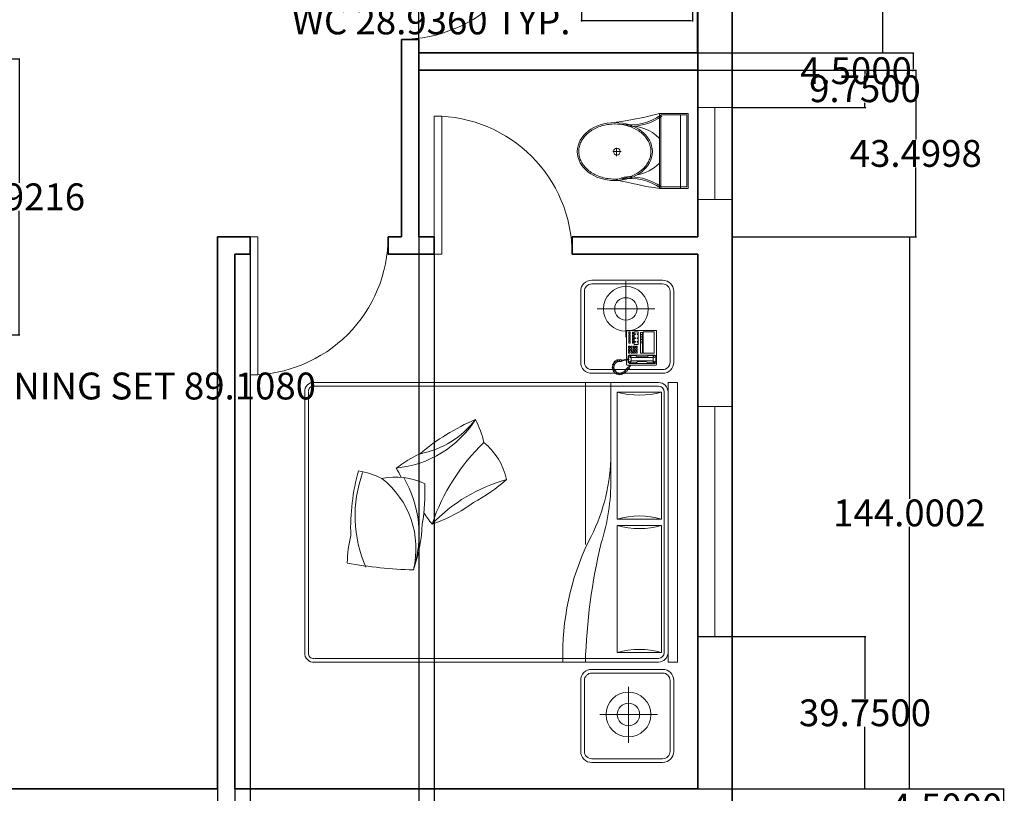
# Model space of a CAD drawing. Units: inches. Extents: x 774 to 2194, y 522 to 1247.
# Tile 3 of 7: x 1035 to 1292, y 668 to 870. Entities that reach past the tile are written whole.
import ezdxf

# ---------------------------------------------------------------- set-up
doc = ezdxf.new("R2010")
doc.units = ezdxf.units.IN
for name, color, linetype, lineweight in [('A-ANNO-DIMS', 2, 'Continuous', 13), ('A-DOOR', 3, 'Continuous', 18), ('A-FLOR-FIXT', 7, 'Continuous', 18), ('A-FURN', 8, 'Continuous', 18), ('A-GLAZ', 4, 'Continuous', 18), ('A-WALL', 7, 'Continuous', 35)]:
    doc.layers.add(name, color=color, linetype=linetype, lineweight=lineweight)
doc.styles.get("Standard").update_dxf_attribs({"font": 'arial.ttf'})
doc.dimstyles.get("Standard").update_dxf_attribs({"dimtxt": 7, "dimasz": 0.18, "dimexe": 0.18, "dimexo": 0.0625, "dimgap": 0.09, "dimtad": 0, "dimtih": 1, "dimtoh": 1, "dimdec": 4, "dimzin": 0, "dimdsep": 46, "dimtxsty": 'Standard', "dimcen": 0.09, "dimadec": 0, "dimazin": 0, "dimtfac": 1, "dimtdec": 4, "dimtofl": 0, "dimtmove": 0, "dimatfit": 3, "dimfxl": 1, "dimtolj": 1, "dimtzin": 0, "dimarcsym": 0})

# ---------------------------------------------------------------- blocks, each defined once
blk = doc.blocks.new('A$C356F0359')
for p, q in [((0.4398, 1.9801), (0.0598, 1.9801)), ((0.4398, 1.9601), (0.0598, 1.9601)), ((0.5489, 2), (2.0492, 2)), ((0.5489, 1.9489), (0.5489, 2)), ((2.0492, 1.9489), (2.0492, 2)), ((2.5283, 1.9801), (2.1483, 1.9801)), ((2.5283, 1.9601), (2.1483, 1.9601)), ((-0.0002, 1.9201), (-0.0002, 1.5401)), ((0.0198, 1.9201), (0.0198, 1.5401)), ((0.4798, 1.5401), (0.4798, 1.9201)), ((0.4998, 1.5401), (0.4998, 1.9201)), ((2.0492, 1.9489), (0.5489, 1.9489)), ((1.998, 1.9289), (0.6001, 1.9289)), ((2.0883, 1.9201), (2.0883, 1.5401)), ((2.1083, 1.9201), (2.1083, 1.5401)), ((2.5683, 1.5401), (2.5683, 1.9201)), ((2.5883, 1.5401), (2.5883, 1.9201)), ((0.1539, 1.5681), (0.1539, 1.8777)), ((0.2725, 1.8879), (0.2702, 1.8856)), ((0.2702, 1.8856), (0.2702, 1.7279)), ((0.2725, 1.8879), (0.4531, 1.8879)), ((0.3913, 1.8753), (0.277, 1.8753)), ((0.277, 1.8753), (0.277, 1.8147)), ((0.3913, 1.8147), (0.3913, 1.8753)), ((0.4016, 1.8787), (0.4062, 1.8845)), ((0.4016, 1.7404), (0.4016, 1.8787)), ((0.4062, 1.881), (0.405, 1.8765)), ((0.405, 1.8765), (0.4153, 1.8662)), ((0.405, 1.8765), (0.405, 1.8456)), ((0.4062, 1.8845), (0.4405, 1.8845)), ((0.4108, 1.8833), (0.4062, 1.881)), ((0.4108, 1.8833), (0.4382, 1.8833)), ((0.4165, 1.8685), (0.4108, 1.8833)), ((0.4153, 1.8662), (0.4165, 1.8685)), ((0.4153, 1.8147), (0.4153, 1.8662)), ((0.4325, 1.8685), (0.4165, 1.8685)), ((0.4325, 1.8685), (0.4382, 1.8833)), ((0.4336, 1.8662), (0.4325, 1.8685)), ((0.4439, 1.8765), (0.4336, 1.8662)), ((0.4336, 1.8147), (0.4336, 1.8662)), ((0.4382, 1.8833), (0.4428, 1.881)), ((0.4405, 1.8845), (0.4462, 1.8787)), ((0.4428, 1.881), (0.4439, 1.8765)), ((0.4439, 1.8765), (0.4439, 1.8456)), ((0.4462, 1.8787), (0.4462, 1.7416)), ((0.4531, 1.8879), (0.4553, 1.8856)), ((0.4553, 1.8856), (0.4553, 1.7279)), ((0.5489, 1.8977), (0.5489, 0.0512)), ((0.5689, 1.8977), (0.5689, 0.0512)), ((2.0292, 0.0512), (2.0292, 1.8977)), ((2.0492, 0.0512), (2.0492, 1.8977)), ((2.3306, 1.5822), (2.3306, 1.8917)), ((0.277, 1.8147), (0.3913, 1.8147)), ((0.3913, 1.8125), (0.2816, 1.8125)), ((0.2816, 1.8125), (0.2816, 1.801)), ((0.2816, 1.801), (0.3913, 1.801)), ((0.2907, 1.8125), (0.2907, 1.801)), ((0.2999, 1.8125), (0.2999, 1.801)), ((0.309, 1.8125), (0.309, 1.801)), ((0.3182, 1.8125), (0.3182, 1.801)), ((0.3273, 1.8125), (0.3273, 1.801)), ((0.3365, 1.8125), (0.3365, 1.801)), ((0.3913, 1.801), (0.3913, 1.8125)), ((0.405, 1.8456), (0.4073, 1.8399)), ((0.4073, 1.8399), (0.4108, 1.8342)), ((0.4108, 1.8342), (0.4119, 1.8262)), ((0.4119, 1.8262), (0.4119, 1.8147)), ((0.4119, 1.793), (0.4119, 1.8147)), ((0.4153, 1.8147), (0.4153, 1.753)), ((0.4336, 1.8147), (0.4336, 1.753)), ((0.4382, 1.8342), (0.4371, 1.8262)), ((0.4371, 1.8262), (0.4371, 1.8147)), ((0.4371, 1.793), (0.4371, 1.8147)), ((0.4416, 1.8399), (0.4382, 1.8342)), ((0.4439, 1.8456), (0.4416, 1.8399)), ((0.277, 1.7885), (0.277, 1.7679)), ((0.3445, 1.7885), (0.277, 1.7885)), ((0.277, 1.7679), (0.3445, 1.7679)), ((0.2782, 1.7622), (0.2782, 1.7576)), ((0.2896, 1.7622), (0.2782, 1.7622)), ((0.2782, 1.7576), (0.2896, 1.7576)), ((0.2782, 1.745), (0.2896, 1.745)), ((0.2782, 1.7382), (0.2782, 1.745)), ((0.2885, 1.7862), (0.2885, 1.7827)), ((0.2919, 1.7862), (0.2885, 1.7862)), ((0.2885, 1.7827), (0.2919, 1.7827)), ((0.2919, 1.7736), (0.2885, 1.7736)), ((0.2885, 1.7736), (0.2885, 1.7702)), ((0.2885, 1.7702), (0.2919, 1.7702)), ((0.2896, 1.7576), (0.2896, 1.7622)), ((0.2896, 1.745), (0.2896, 1.7382)), ((0.2919, 1.7827), (0.2919, 1.7862)), ((0.2919, 1.7702), (0.2919, 1.7736)), ((0.2942, 1.7622), (0.2942, 1.7576)), ((0.3056, 1.7622), (0.2942, 1.7622)), ((0.2942, 1.7576), (0.3056, 1.7576)), ((0.2942, 1.745), (0.3056, 1.745)), ((0.2942, 1.7382), (0.2942, 1.745)), ((0.3056, 1.7576), (0.3056, 1.7622)), ((0.3056, 1.745), (0.3056, 1.7382)), ((0.3125, 1.7862), (0.309, 1.7862)), ((0.309, 1.7862), (0.309, 1.7827)), ((0.309, 1.7827), (0.3125, 1.7827)), ((0.3125, 1.7736), (0.309, 1.7736)), ((0.309, 1.7736), (0.309, 1.7702)), ((0.309, 1.7702), (0.3125, 1.7702)), ((0.3102, 1.7622), (0.3102, 1.7576)), ((0.3216, 1.7622), (0.3102, 1.7622)), ((0.3102, 1.7576), (0.3216, 1.7576)), ((0.3102, 1.745), (0.3216, 1.745)), ((0.3102, 1.7382), (0.3102, 1.745)), ((0.3125, 1.7827), (0.3125, 1.7862)), ((0.3125, 1.7702), (0.3125, 1.7736)), ((0.3216, 1.7576), (0.3216, 1.7622)), ((0.3216, 1.745), (0.3216, 1.7382)), ((0.3376, 1.7622), (0.3262, 1.7622)), ((0.3262, 1.7622), (0.3262, 1.7576)), ((0.3262, 1.7576), (0.3376, 1.7576)), ((0.3262, 1.7382), (0.3262, 1.745)), ((0.3262, 1.745), (0.3376, 1.745)), ((0.333, 1.7862), (0.3296, 1.7862)), ((0.3296, 1.7862), (0.3296, 1.7827)), ((0.3296, 1.7827), (0.333, 1.7827)), ((0.333, 1.7736), (0.3296, 1.7736)), ((0.3296, 1.7736), (0.3296, 1.7702)), ((0.3296, 1.7702), (0.333, 1.7702)), ((0.333, 1.7827), (0.333, 1.7862)), ((0.333, 1.7702), (0.333, 1.7736)), ((0.3376, 1.7576), (0.3376, 1.7622)), ((0.3376, 1.745), (0.3376, 1.7382)), ((0.3445, 1.7679), (0.3445, 1.7885)), ((0.3548, 1.7759), (0.3548, 1.7827)), ((0.3548, 1.7827), (0.3639, 1.7827)), ((0.3639, 1.7759), (0.3548, 1.7759)), ((0.3548, 1.7633), (0.3548, 1.7702)), ((0.3548, 1.7702), (0.3639, 1.7702)), ((0.3639, 1.7633), (0.3548, 1.7633)), ((0.3548, 1.7564), (0.3639, 1.7564)), ((0.3548, 1.7496), (0.3548, 1.7564)), ((0.3639, 1.7496), (0.3548, 1.7496)), ((0.3639, 1.7827), (0.3639, 1.7759)), ((0.3639, 1.7702), (0.3639, 1.7633)), ((0.3639, 1.7564), (0.3639, 1.7496)), ((0.3685, 1.7827), (0.3776, 1.7827)), ((0.3685, 1.7759), (0.3685, 1.7827)), ((0.3776, 1.7759), (0.3685, 1.7759)), ((0.3685, 1.7633), (0.3685, 1.7702)), ((0.3685, 1.7702), (0.3776, 1.7702)), ((0.3776, 1.7633), (0.3685, 1.7633)), ((0.3685, 1.7564), (0.3776, 1.7564)), ((0.3685, 1.7496), (0.3685, 1.7564)), ((0.3776, 1.7496), (0.3685, 1.7496)), ((0.3776, 1.7827), (0.3776, 1.7759)), ((0.3776, 1.7702), (0.3776, 1.7633)), ((0.3776, 1.7564), (0.3776, 1.7496)), ((0.3822, 1.7759), (0.3822, 1.7827)), ((0.3822, 1.7827), (0.3913, 1.7827)), ((0.3913, 1.7759), (0.3822, 1.7759)), ((0.3822, 1.7633), (0.3822, 1.7702)), ((0.3822, 1.7702), (0.3913, 1.7702)), ((0.3913, 1.7633), (0.3822, 1.7633)), ((0.3822, 1.7576), (0.3913, 1.7576)), ((0.3822, 1.7507), (0.3822, 1.7576)), ((0.3913, 1.7507), (0.3822, 1.7507)), ((0.3913, 1.7827), (0.3913, 1.7759)), ((0.3913, 1.7702), (0.3913, 1.7633)), ((0.3913, 1.7576), (0.3913, 1.7507)), ((0.405, 1.7736), (0.4073, 1.7793)), ((0.405, 1.7427), (0.405, 1.7736)), ((0.405, 1.7427), (0.4153, 1.753)), ((0.4073, 1.7793), (0.4108, 1.785)), ((0.4108, 1.785), (0.4119, 1.793)), ((0.4165, 1.7507), (0.4108, 1.7359)), ((0.4153, 1.753), (0.4165, 1.7507)), ((0.4325, 1.7507), (0.4165, 1.7507)), ((0.4336, 1.753), (0.4325, 1.7507)), ((0.4325, 1.7507), (0.4382, 1.7359)), ((0.4439, 1.7427), (0.4336, 1.753)), ((0.4382, 1.785), (0.4371, 1.793)), ((0.4416, 1.7793), (0.4382, 1.785)), ((0.4439, 1.7736), (0.4416, 1.7793)), ((0.4439, 1.7427), (0.4439, 1.7736)), ((0.4622, 1.7459), (0.4553, 1.7484)), ((0.4654, 1.7427), (0.4622, 1.7459)), ((0.3052, 1.7226), (0.0051, 1.7226)), ((0.2702, 1.7279), (0.2725, 1.7256)), ((0.4244, 1.7256), (0.2725, 1.7256)), ((0.2896, 1.7382), (0.2782, 1.7382)), ((0.3056, 1.7382), (0.2942, 1.7382)), ((0.3216, 1.7382), (0.3102, 1.7382)), ((0.3376, 1.7382), (0.3262, 1.7382)), ((0.3548, 1.737), (0.3548, 1.7439)), ((0.3548, 1.7439), (0.3639, 1.7439)), ((0.3639, 1.737), (0.3548, 1.737)), ((0.3639, 1.7439), (0.3639, 1.737)), ((0.3685, 1.737), (0.3685, 1.7439)), ((0.3685, 1.7439), (0.3776, 1.7439)), ((0.3776, 1.737), (0.3685, 1.737)), ((0.3776, 1.7439), (0.3776, 1.737)), ((0.3822, 1.7439), (0.3913, 1.7439)), ((0.3822, 1.737), (0.3822, 1.7439)), ((0.3913, 1.737), (0.3822, 1.737)), ((0.3913, 1.7439), (0.3913, 1.737)), ((0.4073, 1.7347), (0.4016, 1.7404)), ((0.4062, 1.7382), (0.405, 1.7427)), ((0.4108, 1.7359), (0.4062, 1.7382)), ((0.4234, 1.7347), (0.4073, 1.7347)), ((0.4108, 1.7359), (0.4234, 1.7359)), ((0.4233, 1.7393), (0.4235, 1.7294)), ((0.4268, 1.7393), (0.4233, 1.7393)), ((0.4235, 1.7294), (0.4263, 1.7179)), ((0.4263, 1.7179), (0.429, 1.707)), ((0.427, 1.697), (0.4265, 1.6915)), ((0.4265, 1.6915), (0.4332, 1.6903)), ((0.4274, 1.7301), (0.4268, 1.7393)), ((0.427, 1.7359), (0.4382, 1.7359)), ((0.4295, 1.6996), (0.427, 1.697)), ((0.4405, 1.7347), (0.4271, 1.7347)), ((0.429, 1.7227), (0.4274, 1.7301)), ((0.4531, 1.7256), (0.4284, 1.7256)), ((0.429, 1.707), (0.4288, 1.701)), ((0.4288, 1.701), (0.4295, 1.6996)), ((0.4318, 1.7119), (0.429, 1.7227)), ((0.4325, 1.7063), (0.4318, 1.7119)), ((0.4323, 1.7003), (0.4325, 1.7063)), ((0.4364, 1.6973), (0.4323, 1.7003)), ((0.4355, 1.6919), (0.4364, 1.6973)), ((0.4367, 1.6774), (0.4355, 1.6919)), ((0.4382, 1.7359), (0.4428, 1.7382)), ((0.4462, 1.7416), (0.4405, 1.7347)), ((0.4428, 1.7382), (0.4439, 1.7427)), ((0.4553, 1.7279), (0.4531, 1.7256)), ((0.4553, 1.7439), (0.4604, 1.7425)), ((0.4604, 1.7425), (0.465, 1.7388)), ((0.465, 1.7388), (0.4662, 1.7372)), ((0.4678, 1.7405), (0.4654, 1.7427)), ((0.4662, 1.7372), (0.4686, 1.7374)), ((0.4686, 1.7374), (0.4662, 1.735)), ((0.4662, 1.735), (0.4755, 1.7268)), ((0.4721, 1.7421), (0.4678, 1.7405)), ((0.4741, 1.7401), (0.4721, 1.7421)), ((0.4725, 1.7366), (0.4741, 1.7401)), ((0.4753, 1.7388), (0.4725, 1.7366)), ((0.4783, 1.7356), (0.4753, 1.7388)), ((0.4755, 1.7268), (0.4906, 1.7139)), ((0.4759, 1.729), (0.4783, 1.7356)), ((0.4821, 1.7322), (0.4759, 1.729)), ((0.4874, 1.7272), (0.4821, 1.7322)), ((0.4862, 1.7199), (0.4874, 1.7272)), ((0.4914, 1.7231), (0.4862, 1.7199)), ((0.4908, 1.7135), (0.4984, 1.6917)), ((0.4958, 1.7185), (0.4914, 1.7231)), ((0.494, 1.7135), (0.4958, 1.7185)), ((0.501, 1.7142), (0.494, 1.7135)), ((0.4984, 1.6917), (0.4952, 1.6744)), ((0.4964, 1.7047), (0.5031, 1.7072)), ((0.5038, 1.7049), (0.4964, 1.7047)), ((0.5005, 1.695), (0.5054, 1.6996)), ((0.5068, 1.695), (0.5005, 1.695)), ((0.5031, 1.7072), (0.501, 1.7142)), ((0.5054, 1.6996), (0.5038, 1.7049)), ((0.5079, 1.6892), (0.5068, 1.695)), ((2.4819, 1.7366), (2.1818, 1.7366)), ((0.4332, 1.6903), (0.4267, 1.6864)), ((0.4267, 1.6864), (0.4272, 1.6801)), ((0.4272, 1.6801), (0.4346, 1.6794)), ((0.4346, 1.6794), (0.4281, 1.6744)), ((0.4281, 1.6744), (0.4311, 1.669)), ((0.4311, 1.669), (0.4381, 1.6704)), ((0.4381, 1.6704), (0.4348, 1.6639)), ((0.4348, 1.6639), (0.4383, 1.6598)), ((0.4455, 1.6663), (0.4367, 1.6774)), ((0.4383, 1.6598), (0.4436, 1.6637)), ((0.4436, 1.6637), (0.4427, 1.6575)), ((0.4427, 1.6575), (0.4471, 1.6547)), ((0.4577, 1.6598), (0.4455, 1.6663)), ((0.4471, 1.6547), (0.4526, 1.6593)), ((0.4526, 1.6593), (0.4519, 1.6517)), ((0.4519, 1.6517), (0.4568, 1.6503)), ((0.4568, 1.6503), (0.4598, 1.6565)), ((0.4716, 1.6586), (0.4577, 1.6598)), ((0.4598, 1.6565), (0.4626, 1.6503)), ((0.4626, 1.6503), (0.4665, 1.6498)), ((0.4665, 1.6498), (0.4681, 1.6565)), ((0.4681, 1.6565), (0.4707, 1.6491)), ((0.4707, 1.6491), (0.4751, 1.6503)), ((0.485, 1.6644), (0.4716, 1.6586)), ((0.4751, 1.6503), (0.4753, 1.6565)), ((0.4753, 1.6565), (0.4806, 1.6519)), ((0.4806, 1.6519), (0.4843, 1.6538)), ((0.4843, 1.6538), (0.4836, 1.6607)), ((0.4836, 1.6607), (0.4885, 1.6547)), ((0.4952, 1.6744), (0.485, 1.6644)), ((0.4885, 1.6547), (0.4922, 1.6579)), ((0.4922, 1.6579), (0.4894, 1.6642)), ((0.4894, 1.6642), (0.4959, 1.6614)), ((0.4957, 1.6704), (0.5024, 1.6683)), ((0.4989, 1.6642), (0.4957, 1.6704)), ((0.4959, 1.6614), (0.4989, 1.6642)), ((0.5042, 1.673), (0.4987, 1.6792)), ((0.4987, 1.6792), (0.5058, 1.679)), ((0.5008, 1.6871), (0.5079, 1.6892)), ((0.5068, 1.6836), (0.5008, 1.6871)), ((0.5024, 1.6683), (0.5042, 1.673)), ((0.5058, 1.679), (0.5068, 1.6836)), ((0.0598, 1.5001), (0.4398, 1.5001)), ((0.0598, 1.4801), (0.4398, 1.4801)), ((2.1483, 1.5001), (2.5283, 1.5001)), ((2.1483, 1.4801), (2.5283, 1.4801)), ((0.6001, 0.02), (1.998, 0.02)), ((0.6001, 0), (1.998, 0))]:
    blk.add_line(p, q)
at = {"linetype": 'ByBlock'}
for p, q in [((0.6001, 1.9147), (1.282, 1.9147)), ((0.6001, 1.6759), (0.6001, 1.9147)), ((1.282, 1.9147), (1.282, 1.6759)), ((1.3161, 1.9147), (1.998, 1.9147)), ((1.3161, 1.6759), (1.3161, 1.9147)), ((1.998, 1.9147), (1.998, 1.6759)), ((1.0687, 1.6418), (0.5489, 1.6418)), ((1.282, 1.6759), (0.6001, 1.6759)), ((1.998, 1.6759), (1.3161, 1.6759)), ((1.4185, 1.5053), (0.5489, 1.5053))]:
    blk.add_line(p, q, dxfattribs=at)
for centre in [(2.3306, 1.7366), (0.1539, 1.7226)]:
    blk.add_circle(centre, 0.12, dxfattribs=at)
for centre in [(0.1539, 1.7226), (2.3306, 1.7366)]:
    blk.add_circle(centre, 0.06)
for centre, radius, start, end in [((0.0598, 1.9201), 0.06, 90, 180), ((0.0598, 1.9201), 0.04, 90, 180), ((0.4398, 1.9201), 0.06, 0, 90), ((0.4398, 1.9201), 0.04, 0, 90), ((2.1483, 1.9201), 0.06, 90, 180), ((2.1483, 1.9201), 0.04, 90, 180), ((2.5283, 1.9201), 0.06, 0, 90), ((2.5283, 1.9201), 0.04, 0, 90), ((0.6001, 1.8977), 0.0512, 90, 180), ((0.6001, 1.8977), 0.0312, 90, 180), ((1.998, 1.8977), 0.0512, 0, 90), ((1.998, 1.8977), 0.0312, 0, 90), ((0.0598, 1.5401), 0.06, 180, 270), ((0.0598, 1.5401), 0.04, 180, 270), ((0.4398, 1.5401), 0.04, 270, 0), ((0.4398, 1.5401), 0.06, 270, 0), ((2.1483, 1.5401), 0.06, 180, 270), ((2.1483, 1.5401), 0.04, 180, 270), ((2.5283, 1.5401), 0.06, 270, 0), ((2.5283, 1.5401), 0.04, 270, 0), ((1.1471, 0.7332), 0.3575, 102.4782, 140.4625), ((1.9086, 1.3124), 0.8697, 195.336, 226.4193), ((0.3249, 0.4335), 0.9879, 28.4971, 41.0566), ((0.9965, 0.4273), 0.548, 103.2034, 117.0362), ((1.6529, 1.7059), 1.0798, 223.6306, 251.4288), ((0.4451, 0.4375), 0.5655, 5.3391, 57.6895), ((0.4517, 0.5274), 0.4879, 10.6986, 52.6864), ((1.8195, 1.3719), 1.1652, 203.0642, 220.3209), ((0.5617, 0.4344), 0.7874, 18.3527, 36.6851), ((1.4135, 0.487), 0.3575, 154.0418, 192.0262), ((1.1372, -0.3434), 0.9879, 80.0607, 92.6202), ((-0.021, 2.4319), 2.1977, 305.2966, 307.2418), ((1.5949, 0.9312), 0.734, 205.259, 216.9351), ((1.3641, 0.0041), 0.6085, 71.81, 120.1351), ((1.44, 0.1186), 0.4774, 76.1849, 142.0017), ((1.2836, -0.1573), 0.7874, 69.9163, 88.2487), ((-0.6432, 0.628), 2.1977, 349.4884, 358.8054), ((-0.021, 2.4319), 2.1977, 297.9248, 299.3793), ((1.5595, 0.1789), 0.548, 154.767, 168.5998), ((1.2647, 0.9578), 0.6885, 250.2936, 293.6414), ((1.3312, 1.4107), 1.1652, 254.6278, 271.8845), ((1.5368, 0.9609), 0.734, 256.8226, 268.4988), ((0.5943, 0.0454), 0.0458, 172.7599, 277.2401), ((0.5943, 0.0454), 0.0258, 172.7599, 277.2401), ((2.0038, 0.0454), 0.0458, 262.7599, 7.2401), ((2.0038, 0.0454), 0.0258, 262.7599, 7.2401)]:
    blk.add_arc(centre, radius, start, end)
for centre, radius, start, end in [((0.1906, 1.7953), 0.4265, 343.7398, 16.2602), ((1.6914, 1.7953), 0.4265, 163.7398, 196.2602), ((0.9067, 1.7953), 0.4265, 343.7398, 16.2602), ((2.4075, 1.7953), 0.4265, 163.7398, 196.2602), ((0.9303, 0.657), 0.9853, 61.4328, 88.1261), ((1.0826, 0.5712), 1.0706, 72.1966, 90.7418), ((2.1368, 4.5996), 3.0955, 256.4201, 268.3789), ((2.0056, 2.7745), 1.3903, 244.2427, 271.7984)]:
    blk.add_arc(centre, radius, start, end, dxfattribs=at)
blk = doc.blocks.new('A$C31115884')
for p, q in [((283.1, 497.7), (223.4, 497.7)), ((257.5, 466.4), (257.5, 523.2)), ((0, 200), (0, 0)), ((520, 200), (0, 200)), ((10, 190), (10, 10)), ((510, 190), (10, 190)), ((510, 10), (510, 190)), ((520, 0), (520, 200)), ((510, 54.5), (0, 54.5)), ((10, 10), (510, 10)), ((0, 0), (520, 0))]:
    blk.add_line(p, q)
blk.add_circle((255.6, 496.4), 23.6)
for centre, radius, start, end in [((2777.7, -204.6), 2807, 165.4549, 171.71327), ((3237, 905), 2807, 188.28673, 194.5451), ((-294.5, 403.3), 364.7, 324.20913, 9.34987), ((-294.5, 403.3), 374.7, 324.20913, 9.34987), ((139.5, 406.2), 293.5, 315.84364, 2.65635), ((805.8, 403.3), 364.7, 170.65013, 215.79087), ((383.6, 406.2), 293.5, 190.27735, 224.15636), ((805.8, 403.3), 374.7, 179.20365, 215.79087)]:
    blk.add_arc(centre, radius, start, end)
blk.add_ellipse((256.2, 509.9), major_axis=(0, -260.7), ratio=0.772727)
blk.add_open_spline([(256.2, 259.2), (263.1, 259.2), (270, 259.7), (287.8, 262.3), (298.7, 265.1), (319.9, 273.1), (330.2, 278.4), (350.1, 291.1), (359.7, 298.7), (377.7, 315.9), (386.2, 325.5), (401.7, 346.6), (408.8, 358.1), (421.3, 382.5), (426.8, 395.5), (435.9, 422.4), (439.5, 436.4), (444.8, 465.1), (446.5, 479.7), (447.9, 509.2), (447.6, 524), (445, 553.3), (442.7, 567.8), (436.3, 596), (432.1, 609.7), (421.9, 636), (416, 648.6), (402.5, 672.1), (395, 683), (378.6, 703), (369.8, 712.1), (351.1, 728), (341.3, 734.8), (320.9, 746.2), (310.4, 750.7), (288.9, 757.3), (278, 759.4), (256, 761), (245, 760.6), (223.1, 757.2), (212.3, 754.3), (191.1, 746.1), (180.8, 740.7), (160.9, 727.8), (151.4, 720.1), (133.5, 702.7), (125.1, 693), (109.6, 671.7), (102.6, 660.2), (90.2, 635.7), (84.9, 622.7), (76, 595.6), (72.4, 581.6), (67.2, 552.9), (65.6, 538.2), (64.4, 508.8), (64.8, 494), (67.5, 464.7), (69.9, 450.2), (76.6, 422), (80.8, 408.3), (91.1, 382.2), (97.2, 369.7), (110.8, 346.3), (118.4, 335.4), (134.8, 315.6), (143.7, 306.7), (162.4, 290.9), (172.3, 284.2), (192.8, 273), (203.3, 268.6), (224.8, 262.2), (235.8, 260.2), (249.9, 259.3), (253, 259.2), (256.2, 259.2)], degree=3, knots=[0, 0, 0, 0, 0.110105, 0.110105, 0.285049, 0.285049, 0.459994, 0.459994, 0.634938, 0.634938, 0.809882, 0.809882, 0.984827, 0.984827, 1.159771, 1.159771, 1.334715, 1.334715, 1.50966, 1.50966, 1.684604, 1.684604, 1.859549, 1.859549, 2.034493, 2.034493, 2.209437, 2.209437, 2.384382, 2.384382, 2.559326, 2.559326, 2.73427, 2.73427, 2.909215, 2.909215, 3.084159, 3.084159, 3.259103, 3.259103, 3.434048, 3.434048, 3.608992, 3.608992, 3.783936, 3.783936, 3.958881, 3.958881, 4.133825, 4.133825, 4.30877, 4.30877, 4.483714, 4.483714, 4.658658, 4.658658, 4.833603, 4.833603, 5.008547, 5.008547, 5.183491, 5.183491, 5.358436, 5.358436, 5.53338, 5.53338, 5.708324, 5.708324, 5.883269, 5.883269, 6.058213, 6.058213, 6.233158, 6.233158, 6.283185, 6.283185, 6.283185, 6.283185])
blk = doc.blocks.new('*D26')
at = {"layer": 'A-ANNO-DIMS', "color": 0, "lineweight": -2, "transparency": 16777216}
for p, q in [((1211.84, 904.44), (1260.29, 904.44)), ((1260.11, 904.26), (1260.11, 886.35)), ((1260.11, 861.12), (1260.11, 879.02)), ((1211.84, 860.94), (1260.29, 860.94))]:
    blk.add_line(p, q, dxfattribs=at)
at = {"layer": 'A-ANNO-DIMS', "color": 0, "transparency": 16777216}
for points in [[(1260.08, 904.26), (1260.14, 904.26), (1260.11, 904.44)], [(1260.08, 861.12), (1260.14, 861.12), (1260.11, 860.94)]]:
    blk.add_solid(points, dxfattribs=at)
at = {"layer": 'Defpoints', "color": 0, "transparency": 16777216}
for p in [(1211.78, 904.44), (1211.78, 860.94), (1260.11, 860.94)]:
    blk.add_point(p, dxfattribs=at)
at = {"layer": 'A-ANNO-DIMS', "color": 0, "transparency": 16777216, "insert": (1260.11, 882.69), "char_height": 7, "attachment_point": 5}
blk.add_mtext('\\A1;43.5000', dxfattribs=at)
blk = doc.blocks.new('*D27')
at = {"layer": 'A-ANNO-DIMS', "color": 0, "lineweight": -2, "transparency": 16777216}
for p, q in [((1211.84, 860.94), (1268.2, 860.94)), ((1268.02, 860.76), (1268.02, 856.62)), ((1211.84, 856.44), (1268.2, 856.44)), ((1268.02, 856.26), (1267.84, 856.26)), ((1268.02, 856.44), (1268.02, 856.26))]:
    blk.add_line(p, q, dxfattribs=at)
at = {"layer": 'A-ANNO-DIMS', "color": 0, "transparency": 16777216}
for points in [[(1267.99, 860.76), (1268.05, 860.76), (1268.02, 860.94)], [(1267.99, 856.62), (1268.05, 856.62), (1268.02, 856.44)]]:
    blk.add_solid(points, dxfattribs=at)
at = {"layer": 'Defpoints', "color": 0, "transparency": 16777216}
for p in [(1211.78, 860.94), (1211.78, 856.44), (1268.02, 856.44)]:
    blk.add_point(p, dxfattribs=at)
at = {"layer": 'A-ANNO-DIMS', "color": 0, "transparency": 16777216, "insert": (1253.09, 856.26), "char_height": 7, "attachment_point": 5}
blk.add_mtext('\\A1;4.5000', dxfattribs=at)
blk = doc.blocks.new('*D28')
at = {"layer": 'A-ANNO-DIMS', "color": 0, "lineweight": -2, "transparency": 16777216}
for p, q in [((1220.84, 856.44), (1268.86, 856.44)), ((1268.68, 856.26), (1268.68, 838.35)), ((1268.68, 813.12), (1268.68, 831.02)), ((1220.84, 812.94), (1268.86, 812.94))]:
    blk.add_line(p, q, dxfattribs=at)
at = {"layer": 'A-ANNO-DIMS', "color": 0, "transparency": 16777216}
for points in [[(1268.65, 856.26), (1268.71, 856.26), (1268.68, 856.44)], [(1268.65, 813.12), (1268.71, 813.12), (1268.68, 812.94)]]:
    blk.add_solid(points, dxfattribs=at)
at = {"layer": 'Defpoints', "color": 0, "transparency": 16777216}
for p in [(1220.78, 856.44), (1220.78, 812.94), (1268.68, 812.94)]:
    blk.add_point(p, dxfattribs=at)
at = {"layer": 'A-ANNO-DIMS', "color": 0, "transparency": 16777216, "insert": (1268.68, 834.69), "char_height": 7, "attachment_point": 5}
blk.add_mtext('\\A1;43.4998', dxfattribs=at)
blk = doc.blocks.new('*D29')
at = {"layer": 'A-ANNO-DIMS', "color": 0, "lineweight": -2, "transparency": 16777216}
for p, q in [((1220.84, 812.94), (1267.19, 812.94)), ((1267.01, 812.76), (1267.01, 744.6)), ((1267.01, 669.12), (1267.01, 737.27)), ((1220.84, 668.94), (1267.19, 668.94))]:
    blk.add_line(p, q, dxfattribs=at)
at = {"layer": 'A-ANNO-DIMS', "color": 0, "transparency": 16777216}
for points in [[(1266.98, 812.76), (1267.04, 812.76), (1267.01, 812.94)], [(1266.98, 669.12), (1267.04, 669.12), (1267.01, 668.94)]]:
    blk.add_solid(points, dxfattribs=at)
at = {"layer": 'Defpoints', "color": 0, "transparency": 16777216}
for p in [(1220.78, 812.94), (1220.78, 668.94), (1267.01, 668.94)]:
    blk.add_point(p, dxfattribs=at)
at = {"layer": 'A-ANNO-DIMS', "color": 0, "transparency": 16777216, "insert": (1267.01, 740.94), "char_height": 7, "attachment_point": 5}
blk.add_mtext('\\A1;144.0002', dxfattribs=at)
blk = doc.blocks.new('*D30')
at = {"layer": 'A-ANNO-DIMS', "color": 0, "lineweight": -2, "transparency": 16777216}
for p, q in [((1211.84, 668.94), (1291.77, 668.94)), ((1291.59, 668.76), (1291.59, 664.62)), ((1211.84, 664.44), (1291.77, 664.44)), ((1291.59, 664.26), (1291.41, 664.26)), ((1291.59, 664.44), (1291.59, 664.26))]:
    blk.add_line(p, q, dxfattribs=at)
at = {"layer": 'A-ANNO-DIMS', "color": 0, "transparency": 16777216}
for points in [[(1291.56, 668.76), (1291.62, 668.76), (1291.59, 668.94)], [(1291.56, 664.62), (1291.62, 664.62), (1291.59, 664.44)]]:
    blk.add_solid(points, dxfattribs=at)
at = {"layer": 'Defpoints', "color": 0, "transparency": 16777216}
for p in [(1211.78, 668.94), (1211.78, 664.44), (1291.59, 664.44)]:
    blk.add_point(p, dxfattribs=at)
at = {"layer": 'A-ANNO-DIMS', "color": 0, "transparency": 16777216, "insert": (1276.66, 664.26), "char_height": 7, "attachment_point": 5}
blk.add_mtext('\\A1;4.5000', dxfattribs=at)
blk = doc.blocks.new('DOOR-SWING-36IN')
blk.add_line((36, 0), (36, 2))
blk.add_lwpolyline([(36, 2), (0, 2), (0, 0), (36, 0)], close=True)
blk.add_arc((36, 0), 36, 90, 180)
blk = doc.blocks.new('WIN-60IN-EXT')
for p, q in [((0, 0), (0, 9)), ((60, 0), (60, 9)), ((0, 4.5), (60, 4.5))]:
    blk.add_line(p, q)
blk = doc.blocks.new('WIN-24IN-EXT')
for p, q in [((0, 0), (0, 9)), ((24, 0), (24, 9)), ((0, 4.5), (24, 4.5))]:
    blk.add_line(p, q)
blk = doc.blocks.new('*D44')
at = {"layer": 'A-ANNO-DIMS', "color": 0, "lineweight": -2, "transparency": 16777216}
for p, q in [((1181.45, 873.52), (1181.45, 869.06)), ((1210.39, 873.52), (1210.39, 869.06)), ((1181.45, 869.24), (1181.27, 869.24)), ((1210.21, 869.24), (1181.63, 869.24))]:
    blk.add_line(p, q, dxfattribs=at)
at = {"layer": 'A-ANNO-DIMS', "color": 0, "transparency": 16777216}
for points in [[(1181.63, 869.27), (1181.63, 869.21), (1181.45, 869.24)], [(1210.21, 869.27), (1210.21, 869.21), (1210.39, 869.24)]]:
    blk.add_solid(points, dxfattribs=at)
at = {"layer": 'Defpoints', "color": 0, "transparency": 16777216}
for p in [(1181.45, 873.58), (1210.39, 873.58), (1181.45, 869.24)]:
    blk.add_point(p, dxfattribs=at)
at = {"layer": 'A-ANNO-DIMS', "color": 0, "transparency": 16777216, "insert": (1142.26, 869.24), "char_height": 7, "attachment_point": 5}
blk.add_mtext('\\A1;WC 28.9360 TYP.', dxfattribs=at)
blk = doc.blocks.new('*D46')
at = {"layer": 'A-ANNO-DIMS', "color": 0, "lineweight": -2, "transparency": 16777216}
for p, q in [((932.28, 787.34), (932.28, 773.85)), ((1021.39, 787.34), (1021.39, 773.85)), ((932.46, 774.03), (1021.21, 774.03)), ((1021.39, 774.03), (1021.57, 774.03))]:
    blk.add_line(p, q, dxfattribs=at)
at = {"layer": 'A-ANNO-DIMS', "color": 0, "transparency": 16777216}
for points in [[(932.46, 774.06), (932.46, 774), (932.28, 774.03)], [(1021.21, 774.06), (1021.21, 774), (1021.39, 774.03)]]:
    blk.add_solid(points, dxfattribs=at)
at = {"layer": 'Defpoints', "color": 0, "transparency": 16777216}
for p in [(932.28, 787.4), (1021.39, 787.4), (1021.39, 774.03)]:
    blk.add_point(p, dxfattribs=at)
at = {"layer": 'A-ANNO-DIMS', "color": 0, "transparency": 16777216, "insert": (1068.06, 774.03), "char_height": 7, "attachment_point": 5}
blk.add_mtext('\\A1;DINING SET 89.1080', dxfattribs=at)
blk = doc.blocks.new('*D47')
at = {"layer": 'A-ANNO-DIMS', "color": 0, "lineweight": -2, "transparency": 16777216}
for p, q in [((1021.45, 859.32), (1034.94, 859.32)), ((1034.76, 859.14), (1034.76, 827.02)), ((1034.76, 787.58), (1034.76, 819.7)), ((1021.45, 787.4), (1034.94, 787.4))]:
    blk.add_line(p, q, dxfattribs=at)
at = {"layer": 'A-ANNO-DIMS', "color": 0, "transparency": 16777216}
for points in [[(1034.73, 859.14), (1034.79, 859.14), (1034.76, 859.32)], [(1034.73, 787.58), (1034.79, 787.58), (1034.76, 787.4)]]:
    blk.add_solid(points, dxfattribs=at)
at = {"layer": 'Defpoints', "color": 0, "transparency": 16777216}
for p in [(1021.39, 859.32), (1034.76, 859.32), (1021.39, 787.4)]:
    blk.add_point(p, dxfattribs=at)
at = {"layer": 'A-ANNO-DIMS', "color": 0, "transparency": 16777216, "insert": (1034.76, 823.36), "char_height": 7, "attachment_point": 5}
blk.add_mtext('\\A1;71.9216', dxfattribs=at)
blk = doc.blocks.new('*D50')
at = {"layer": 'A-ANNO-DIMS', "color": 0, "lineweight": -2, "transparency": 16777216}
for p, q in [((1139.03, 861), (1139.03, 1085.52)), ((1139.21, 1085.34), (1158.11, 1085.34)), ((1211.6, 1085.34), (1192.7, 1085.34)), ((1211.78, 861), (1211.78, 1085.52))]:
    blk.add_line(p, q, dxfattribs=at)
at = {"layer": 'A-ANNO-DIMS', "color": 0, "transparency": 16777216}
for points in [[(1139.21, 1085.37), (1139.21, 1085.31), (1139.03, 1085.34)], [(1211.6, 1085.37), (1211.6, 1085.31), (1211.78, 1085.34)]]:
    blk.add_solid(points, dxfattribs=at)
at = {"layer": 'Defpoints', "color": 0, "transparency": 16777216}
for p in [(1211.78, 1085.34), (1139.03, 860.94), (1211.78, 860.94)]:
    blk.add_point(p, dxfattribs=at)
at = {"layer": 'A-ANNO-DIMS', "color": 0, "transparency": 16777216, "insert": (1175.41, 1085.34), "char_height": 7, "attachment_point": 5}
blk.add_mtext('\\A1;72.7500', dxfattribs=at)
blk = doc.blocks.new('*D55')
at = {"layer": 'A-ANNO-DIMS', "color": 0, "lineweight": -2, "transparency": 16777216}
for p, q in [((869.78, 668.88), (869.78, 526.86)), ((1086.53, 668.88), (1086.53, 526.86)), ((869.96, 527.04), (958.05, 527.04)), ((1086.35, 527.04), (998.26, 527.04))]:
    blk.add_line(p, q, dxfattribs=at)
at = {"layer": 'A-ANNO-DIMS', "color": 0, "transparency": 16777216}
for points in [[(869.96, 527.07), (869.96, 527.01), (869.78, 527.04)], [(1086.35, 527.07), (1086.35, 527.01), (1086.53, 527.04)]]:
    blk.add_solid(points, dxfattribs=at)
at = {"layer": 'Defpoints', "color": 0, "transparency": 16777216}
for p in [(869.78, 668.94), (1086.53, 668.94), (1086.53, 527.04)]:
    blk.add_point(p, dxfattribs=at)
at = {"layer": 'A-ANNO-DIMS', "color": 0, "transparency": 16777216, "insert": (978.16, 527.04), "char_height": 7, "attachment_point": 5}
blk.add_mtext('\\A1;216.7500', dxfattribs=at)
blk = doc.blocks.new('*D64')
at = {"layer": 'A-ANNO-DIMS', "color": 0, "lineweight": -2, "transparency": 16777216}
for p, q in [((1211.84, 708.69), (1255.61, 708.69)), ((1255.43, 708.51), (1255.43, 692.48)), ((1255.43, 669.12), (1255.43, 685.15)), ((1211.84, 668.94), (1255.61, 668.94))]:
    blk.add_line(p, q, dxfattribs=at)
at = {"layer": 'A-ANNO-DIMS', "color": 0, "transparency": 16777216}
for points in [[(1255.4, 708.51), (1255.46, 708.51), (1255.43, 708.69)], [(1255.4, 669.12), (1255.46, 669.12), (1255.43, 668.94)]]:
    blk.add_solid(points, dxfattribs=at)
at = {"layer": 'Defpoints', "color": 0, "transparency": 16777216}
for p in [(1211.78, 708.69), (1255.43, 708.69), (1211.78, 668.94)]:
    blk.add_point(p, dxfattribs=at)
at = {"layer": 'A-ANNO-DIMS', "color": 0, "transparency": 16777216, "insert": (1255.43, 688.81), "char_height": 7, "attachment_point": 5}
blk.add_mtext('\\A1;39.7500', dxfattribs=at)
blk = doc.blocks.new('*D66')
at = {"layer": 'A-ANNO-DIMS', "color": 0, "lineweight": -2, "transparency": 16777216}
for p, q in [((1211.84, 856.44), (1255.61, 856.44)), ((1255.43, 856.26), (1255.43, 855.23)), ((1255.43, 846.87), (1255.43, 847.9)), ((1220.84, 846.69), (1255.61, 846.69))]:
    blk.add_line(p, q, dxfattribs=at)
at = {"layer": 'A-ANNO-DIMS', "color": 0, "transparency": 16777216}
for points in [[(1255.4, 856.26), (1255.46, 856.26), (1255.43, 856.44)], [(1255.4, 846.87), (1255.46, 846.87), (1255.43, 846.69)]]:
    blk.add_solid(points, dxfattribs=at)
at = {"layer": 'Defpoints', "color": 0, "transparency": 16777216}
for p in [(1211.78, 856.44), (1255.43, 856.44), (1220.78, 846.69)]:
    blk.add_point(p, dxfattribs=at)
at = {"layer": 'A-ANNO-DIMS', "color": 0, "transparency": 16777216, "insert": (1255.43, 851.56), "char_height": 7, "attachment_point": 5}
blk.add_mtext('\\A1;9.7500', dxfattribs=at)
blk = doc.blocks.new('*D71')
at = {"layer": 'A-ANNO-DIMS', "color": 0, "lineweight": -2, "transparency": 16777216}
for p, q in [((1139.03, 812.87), (1139.03, 526.86)), ((1143.03, 812.87), (1143.03, 526.86)), ((1139.21, 527.04), (1142.85, 527.04)), ((1143.03, 527.04), (1143.21, 527.04))]:
    blk.add_line(p, q, dxfattribs=at)
at = {"layer": 'A-ANNO-DIMS', "color": 0, "transparency": 16777216}
for points in [[(1139.21, 527.07), (1139.21, 527.01), (1139.03, 527.04)], [(1142.85, 527.07), (1142.85, 527.01), (1143.03, 527.04)]]:
    blk.add_solid(points, dxfattribs=at)
at = {"layer": 'Defpoints', "color": 0, "transparency": 16777216}
for p in [(1139.03, 812.94), (1143.03, 812.94), (1143.03, 527.04)]:
    blk.add_point(p, dxfattribs=at)
at = {"layer": 'A-ANNO-DIMS', "color": 0, "transparency": 16777216, "insert": (1157.96, 527.04), "char_height": 7, "attachment_point": 5}
blk.add_mtext('\\A1;4.0000', dxfattribs=at)
blk = doc.blocks.new('*D74')
at = {"layer": 'A-ANNO-DIMS', "color": 0, "lineweight": -2, "transparency": 16777216}
for p, q in [((1091.03, 808.38), (1091.03, 526.86)), ((1095.03, 808.38), (1095.03, 526.86)), ((1091.21, 527.04), (1094.85, 527.04)), ((1095.03, 527.04), (1095.21, 527.04))]:
    blk.add_line(p, q, dxfattribs=at)
at = {"layer": 'A-ANNO-DIMS', "color": 0, "transparency": 16777216}
for points in [[(1091.21, 527.07), (1091.21, 527.01), (1091.03, 527.04)], [(1094.85, 527.07), (1094.85, 527.01), (1095.03, 527.04)]]:
    blk.add_solid(points, dxfattribs=at)
at = {"layer": 'Defpoints', "color": 0, "transparency": 16777216}
for p in [(1091.03, 808.44), (1095.03, 808.44), (1095.03, 527.04)]:
    blk.add_point(p, dxfattribs=at)
at = {"layer": 'A-ANNO-DIMS', "color": 0, "transparency": 16777216, "insert": (1109.96, 527.04), "char_height": 7, "attachment_point": 5}
blk.add_mtext('\\A1;4.0000', dxfattribs=at)

msp = doc.modelspace()

# ---------------------------------------------------------------- linework, layer by layer
at = {"layer": 'A-WALL'}
for p, q in [((1220.78103, 570.6875), (1220.78103, 1050.6875)), ((1220.78103, 906.6875), (1220.78103, 810.6875)), ((1211.78103, 904.4375), (1211.78103, 860.9375)), ((1211.78103, 812.93733), (1211.78103, 904.4375)), ((1134.53103, 864.4375), (1139.03103, 864.4375)), ((1134.53103, 864.4375), (1134.53103, 812.93589)), ((1139.03103, 864.4375), (1139.03103, 812.93598)), ((1139.03103, 860.9375), (1211.78103, 860.9375)), ((1139.03103, 856.4375), (1211.78103, 856.4375)), ((1211.78103, 812.93733), (1211.78103, 856.4375)), ((1086.53103, 812.935), (1091.03094, 812.93508)), ((1086.53103, 812.935), (1086.53103, 668.9375)), ((1095.03094, 812.93508), (1091.03094, 812.935)), ((1095.03103, 808.4375), (1095.03094, 812.93508)), ((1131.03103, 808.4375), (1131.03094, 812.93508)), ((1131.03094, 812.93508), (1134.53103, 812.93508)), ((1143.03103, 812.93598), (1139.03103, 812.93598)), ((1143.03103, 812.93598), (1143.03103, 808.4375)), ((1179.03103, 812.93598), (1211.78103, 812.93733)), ((1179.03103, 812.93598), (1179.03103, 808.4375)), ((1091.03103, 808.4375), (1095.03103, 808.4375)), ((1091.03103, 808.4375), (1091.03103, 668.9375)), ((1131.03103, 808.4375), (1143.03103, 808.4375)), ((1179.03103, 808.4375), (1211.78103, 808.4375)), ((1211.78103, 668.9375), (1211.78103, 808.4375)), ((1211.78103, 668.9375), (1211.78103, 808.4375)), ((1010.53103, 668.9375), (1086.53103, 668.9375)), ((1091.03103, 668.9375), (1211.78103, 668.9375))]:
    msp.add_line(p, q, dxfattribs=at)

# ---------------------------------------------------------------- block references
at = {"layer": 'A-DOOR'}
for p, rotation in [((1170.53061, 900.43709), 180), ((1143.03144, 844.43708), 270.0000000000004)]:
    msp.add_blockref('DOOR-SWING-36IN', p, dxfattribs=dict(at, rotation=rotation))
at = {"layer": 'A-DOOR', "extrusion": (0, 0, -1), "zscale": -1, "rotation": 90.00000000000018}
msp.add_blockref('DOOR-SWING-36IN', (-1095.03136, 776.9355), dxfattribs=at)
at = {"layer": 'A-FLOR-FIXT', "xscale": 0.0375513777956547, "yscale": 0.0375513777956547, "zscale": 0.0375513777956547, "rotation": 89.99999999999999}
msp.add_blockref('A$C31115884', (1209.32804, 825.55767), dxfattribs=at)
at = {"layer": 'A-FURN', "xscale": 48.60038017161549, "yscale": 48.60038017161549, "zscale": 48.60038017161549, "rotation": 270}
msp.add_blockref('A$C356F0359', (1109.33091, 801.62985), dxfattribs=at)
at = {"layer": 'A-GLAZ'}
for name, p, rotation in [('WIN-24IN-EXT', (1211.78152, 846.68775), 269.9999999999983), ('WIN-60IN-EXT', (1220.78053, 708.68748), 90)]:
    msp.add_blockref(name, p, dxfattribs=dict(at, rotation=rotation))

# ---------------------------------------------------------------- dimensions: what is measured, and where the dimension line sits
at = {"layer": 'A-ANNO-DIMS'}
for base, p1, p2, picture, middle in [((1211.78103, 1085.3375), (1139.03103, 860.9375), (1211.78103, 860.9375), '*D50', (1175.40603, 1085.3375)), ((1143.03103, 527.0375), (1139.03103, 812.93598), (1143.03103, 812.93598), '*D71', (1157.95996, 527.0375)), ((1095.03103, 527.0375), (1091.03103, 808.4375), (1095.03103, 808.4375), '*D74', (1109.95996, 527.0375)), ((1086.53103, 527.0375), (869.78103, 668.9375), (1086.53103, 668.9375), '*D55', (978.15603, 527.0375))]:
    dim = msp.add_linear_dim(base=base, p1=p1, p2=p2, dimstyle='Standard', override={"dimdec": 4, "dimlfac": 1, "dimrnd": 0, "dimzin": 0, "dimdsep": 46, "dimlunit": 2}, dxfattribs=at)
    dim.commit()
    dim.dimension.update_dxf_attribs({"geometry": picture, "text_midpoint": middle})
for base, p1, p2, override, picture, middle in [((1260.11063, 860.9375), (1211.78103, 904.4375), (1211.78103, 860.9375), {"dimclrd": 0, "dimclre": 0, "dimclrt": 0}, '*D26', (1260.11063, 882.6875)), ((1268.0163, 856.4375), (1211.78103, 860.9375), (1211.78103, 856.4375), {"dimclrd": 0, "dimclre": 0, "dimclrt": 0}, '*D27', (1253.08736, 856.2575)), ((1034.75683, 859.32037), (1021.39063, 787.39874), (1021.39063, 859.32037), {"dimdec": 4, "dimlfac": 1, "dimrnd": 0, "dimzin": 0, "dimdsep": 46, "dimlunit": 2}, '*D47', (1034.75683, 823.35956)), ((1255.43103, 856.4375), (1220.78103, 846.6875), (1211.78103, 856.4375), {"dimdec": 4, "dimlfac": 1, "dimrnd": 0, "dimzin": 0, "dimdsep": 46, "dimlunit": 2}, '*D66', (1255.43103, 851.5625)), ((1268.68032, 812.93771), (1220.78103, 856.4375), (1220.78103, 812.93771), {"dimclrd": 0, "dimclre": 0, "dimclrt": 0}, '*D28', (1268.68032, 834.68761)), ((1267.01333, 668.9375), (1220.78103, 812.93771), (1220.78103, 668.9375), {"dimclrd": 0, "dimclre": 0, "dimclrt": 0}, '*D29', (1267.01333, 740.93761)), ((1255.43103, 708.6875), (1211.78103, 668.9375), (1211.78103, 708.6875), {"dimdec": 4, "dimlfac": 1, "dimrnd": 0, "dimzin": 0, "dimdsep": 46, "dimlunit": 2}, '*D64', (1255.43103, 688.8125)), ((1291.5904, 664.4375), (1211.78103, 668.9375), (1211.78103, 664.4375), {"dimclrd": 0, "dimclre": 0, "dimclrt": 0}, '*D30', (1276.66146, 664.2575))]:
    dim = msp.add_linear_dim(base=base, p1=p1, p2=p2, angle=90, dimstyle='Standard', override=override, dxfattribs=at)
    dim.commit()
    dim.dimension.update_dxf_attribs({"geometry": picture, "text_midpoint": middle})
dim = msp.add_linear_dim(base=(1181.45237, 869.24227), p1=(1210.38834, 873.58267), p2=(1181.45237, 873.58267), angle=180, text='WC <> TYP.', dimstyle='Standard', override={"dimdec": 4, "dimlfac": 1, "dimrnd": 0, "dimzin": 0, "dimdsep": 46, "dimlunit": 2}, dxfattribs=at)
dim.commit()
dim.dimension.update_dxf_attribs({"geometry": '*D44', "text_midpoint": (1142.26218, 869.24227)})
dim = msp.add_linear_dim(base=(1021.39063, 774.03254), p1=(932.2826, 787.39874), p2=(1021.39063, 787.39874), text='DINING SET <>', dimstyle='Standard', override={"dimdec": 4, "dimlfac": 1, "dimrnd": 0, "dimzin": 0, "dimdsep": 46, "dimlunit": 2}, dxfattribs=at)
dim.commit()
dim.dimension.update_dxf_attribs({"geometry": '*D46', "text_midpoint": (1068.06308, 774.03254)})

doc.saveas('drawing.dxf')
